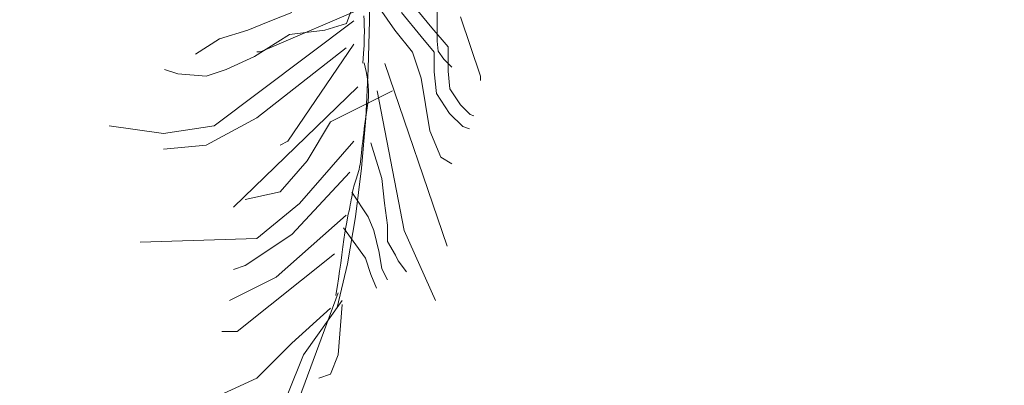
# Model space of a CAD drawing. Units: millimetres. Extents: x 595116 to 630915, y 909473 to 920225.
# Tile 57 of 134: x 629601.67 to 629608.928, y 919288.018 to 919290.711. Entities that reach past the tile are written whole.
import ezdxf

# ---------------------------------------------------------------- set-up
doc = ezdxf.new("R2010")
doc.units = ezdxf.units.MM
doc.layers.add('Dimension', color=3, linetype='Continuous', lineweight=18)
doc.layers.add('L-PLNT', color=85, linetype='Continuous', lineweight=13)
doc.styles.get("Standard").update_dxf_attribs({"font": 'arial.ttf'})
doc.dimstyles.new('ISO-25', dxfattribs={"dimtxt": 9, "dimasz": 6, "dimexe": 1.25, "dimexo": 0.625, "dimtad": 1, "dimlunit": 4, "dimtxsty": 'Standard', "dimcen": 2.5, "dimadec": 0, "dimazin": 0, "dimtfac": 1, "dimtmove": 0, "dimatfit": 3, "dimfxl": 1, "dimarcsym": 0})

# ---------------------------------------------------------------- blocks, each defined once
blk = doc.blocks.new('A$C4FB75ABC')
for p, q in [((3.3496, 1.0323), (3.3109, 0.9247)), ((3.3557, 1.0207), (3.3558, 0.9307)), ((3.3555, 0.9604), (3.142, 0.8689)), ((3.3755, 0.9548), (3.4056, 0.9118)), ((3.4413, 0.9609), (3.4779, 0.9162)), ((3.4889, 0.9539), (3.4889, 0.8899)), ((3.325, 0.9299), (3.0505, 0.7241)), ((3.1171, 0.9118), (3.1602, 0.929)), ((3.1602, 0.929), (3.2032, 0.9462)), ((3.3449, 0.9399), (3.3453, 0.931)), ((3.3453, 0.931), (3.3456, 0.921)), ((3.3558, 0.9307), (3.3535, 0.836)), ((3.4185, 0.9462), (3.4573, 0.8989)), ((3.5348, 0.9376), (3.5735, 0.8214)), ((3.0612, 0.8946), (3.1171, 0.9118)), ((3.2678, 0.9118), (3.1989, 0.9032)), ((3.3109, 0.9247), (3.2678, 0.9118)), ((3.3456, 0.921), (3.3457, 0.9097)), ((3.3457, 0.9097), (3.3456, 0.8969)), ((3.4056, 0.9118), (3.44, 0.8687)), ((3.4779, 0.9162), (3.5101, 0.8787)), ((3.0138, 0.8644), (3.0612, 0.8946)), ((3.1989, 0.9032), (3.1301, 0.8601)), ((3.3456, 0.8969), (3.3451, 0.8822)), ((3.4573, 0.8989), (3.4831, 0.8687)), ((3.4889, 0.8899), (3.4909, 0.8704)), ((3.3098, 0.8766), (3.1344, 0.7394)), ((3.325, 0.8842), (3.1954, 0.6936)), ((3.3451, 0.8822), (3.3441, 0.8655)), ((3.4909, 0.8704), (3.5015, 0.8546)), ((3.5101, 0.8787), (3.5101, 0.8314)), ((3.1301, 0.8601), (3.0741, 0.8343)), ((3.142, 0.8689), (3.1344, 0.8689)), ((3.3441, 0.8655), (3.3424, 0.8466)), ((3.44, 0.8687), (3.4573, 0.8171)), ((3.4831, 0.8687), (3.4831, 0.83)), ((3.5015, 0.8546), (3.5172, 0.8388)), ((2.9794, 0.8257), (2.9535, 0.8343)), ((3.0741, 0.8343), (3.0353, 0.8214)), ((3.3453, 0.8472), (3.3494, 0.8306)), ((3.3535, 0.836), (3.3484, 0.7387)), ((3.386, 0.8461), (3.508, 0.4878)), ((3.0353, 0.8214), (2.9794, 0.8257)), ((3.3494, 0.8306), (3.3521, 0.8161)), ((3.3521, 0.8161), (3.3535, 0.8034)), ((3.4573, 0.8171), (3.4659, 0.7655)), ((3.4831, 0.83), (3.4874, 0.787)), ((3.5101, 0.8314), (3.5136, 0.7963)), ((3.5735, 0.8214), (3.5735, 0.8128)), ((3.3326, 0.8003), (3.0886, 0.5641)), ((3.3535, 0.8034), (3.354, 0.7921)), ((3.5136, 0.7963), (3.5342, 0.7654)), ((3.4013, 0.7927), (3.2793, 0.7317)), ((3.3537, 0.7819), (3.3529, 0.7725)), ((3.354, 0.7921), (3.3537, 0.7819)), ((3.3708, 0.7927), (3.4242, 0.5183)), ((3.4874, 0.787), (3.5132, 0.7482)), ((3.3503, 0.7547), (3.349, 0.7457)), ((3.3517, 0.7635), (3.3503, 0.7547)), ((3.3529, 0.7725), (3.3517, 0.7635)), ((3.4659, 0.7655), (3.4745, 0.7138)), ((3.5342, 0.7654), (3.5536, 0.746)), ((3.1344, 0.7394), (3.0352, 0.686)), ((3.3484, 0.7387), (3.34, 0.641)), ((3.3478, 0.7367), (3.3466, 0.7276)), ((3.349, 0.7457), (3.3478, 0.7367)), ((3.5132, 0.7482), (3.5391, 0.7224)), ((3.5536, 0.746), (3.5605, 0.7437)), ((2.9513, 0.7089), (2.8446, 0.7241)), ((3.0505, 0.7241), (2.9513, 0.7089)), ((3.2793, 0.7317), (3.2335, 0.6555)), ((3.3455, 0.7186), (3.3445, 0.7097)), ((3.3466, 0.7276), (3.3455, 0.7186)), ((3.5391, 0.7224), (3.552, 0.7181)), ((3.3435, 0.7011), (3.3426, 0.6929)), ((3.3445, 0.7097), (3.3435, 0.7011)), ((3.4745, 0.7138), (3.496, 0.6622)), ((3.0352, 0.686), (2.9513, 0.6784)), ((3.1954, 0.6936), (3.1801, 0.686)), ((3.325, 0.6936), (3.2182, 0.5717)), ((3.341, 0.6779), (3.3402, 0.6711)), ((3.3417, 0.6851), (3.341, 0.6779)), ((3.3426, 0.6929), (3.3417, 0.6851)), ((3.3586, 0.6905), (3.3801, 0.6206)), ((3.3388, 0.6589), (3.338, 0.6533)), ((3.3395, 0.6648), (3.3388, 0.6589)), ((3.3402, 0.6711), (3.3395, 0.6648)), ((3.496, 0.6622), (3.5175, 0.6493)), ((3.2335, 0.6555), (3.1801, 0.5945)), ((3.34, 0.641), (3.3282, 0.5451)), ((3.3353, 0.6385), (3.3341, 0.634)), ((3.3363, 0.6432), (3.3353, 0.6385)), ((3.3372, 0.6481), (3.3363, 0.6432)), ((3.338, 0.6533), (3.3372, 0.6481)), ((3.3174, 0.6327), (3.203, 0.5107)), ((3.3303, 0.6215), (3.3289, 0.6175)), ((3.3316, 0.6256), (3.3303, 0.6215)), ((3.3329, 0.6297), (3.3316, 0.6256)), ((3.3341, 0.634), (3.3329, 0.6297)), ((3.3801, 0.6206), (3.3855, 0.5721)), ((3.3242, 0.6014), (3.3233, 0.5973)), ((3.3252, 0.6055), (3.3242, 0.6014)), ((3.3264, 0.6095), (3.3252, 0.6055)), ((3.3276, 0.6135), (3.3264, 0.6095)), ((3.3289, 0.6175), (3.3276, 0.6135)), ((3.1801, 0.5945), (3.1115, 0.5793)), ((3.3208, 0.584), (3.32, 0.5792)), ((3.3216, 0.5886), (3.3208, 0.584)), ((3.3209, 0.5936), (3.3532, 0.5452)), ((3.3225, 0.593), (3.3216, 0.5886)), ((3.3233, 0.5973), (3.3225, 0.593)), ((3.2182, 0.5717), (3.1344, 0.5031)), ((3.3169, 0.5634), (3.3156, 0.5574)), ((3.3181, 0.5689), (3.3169, 0.5634)), ((3.3191, 0.5742), (3.3181, 0.5689)), ((3.32, 0.5792), (3.3191, 0.5742)), ((3.3855, 0.5721), (3.3909, 0.5291)), ((3.3098, 0.5488), (3.1725, 0.4269)), ((3.3127, 0.5432), (3.3111, 0.5347)), ((3.3282, 0.5451), (3.3124, 0.4531)), ((3.3142, 0.5507), (3.3127, 0.5432)), ((3.3156, 0.5574), (3.3142, 0.5507)), ((3.3532, 0.5452), (3.364, 0.5183)), ((3.3047, 0.5237), (3.3478, 0.4645)), ((3.3093, 0.5249), (3.3075, 0.5137)), ((3.3111, 0.5347), (3.3093, 0.5249)), ((3.3909, 0.5291), (3.3909, 0.4968)), ((3.1344, 0.5031), (2.9056, 0.4955)), ((3.203, 0.5107), (3.1115, 0.4497)), ((3.3075, 0.5137), (3.3055, 0.5008)), ((3.364, 0.5183), (3.3747, 0.4753)), ((3.4242, 0.5183), (3.4852, 0.3811)), ((3.3034, 0.4863), (3.3013, 0.4707)), ((3.3055, 0.5008), (3.3034, 0.4863)), ((3.3909, 0.4968), (3.407, 0.4699)), ((3.2869, 0.4726), (3.0962, 0.3201)), ((3.3013, 0.4707), (3.2992, 0.4546)), ((3.3478, 0.4645), (3.3586, 0.4322)), ((3.3747, 0.4753), (3.3801, 0.443)), ((3.407, 0.4699), (3.4124, 0.4591)), ((3.1115, 0.4497), (3.0886, 0.4421)), ((3.3124, 0.4531), (3.2923, 0.3674)), ((3.2992, 0.4546), (3.297, 0.4387)), ((3.4124, 0.4591), (3.4286, 0.4376)), ((3.1725, 0.4269), (3.081, 0.3811)), ((3.297, 0.4387), (3.2949, 0.4237)), ((3.3586, 0.4322), (3.3693, 0.4053)), ((3.3801, 0.443), (3.3909, 0.4214)), ((3.2929, 0.4103), (3.2911, 0.3992)), ((3.2949, 0.4237), (3.2929, 0.4103)), ((3.2945, 0.3964), (3.2182, 0.1906)), ((3.2911, 0.3992), (3.2894, 0.3911)), ((3.3021, 0.3811), (3.2259, 0.2744)), ((3.3021, 0.3735), (3.2945, 0.2744)), ((3.2793, 0.3659), (3.203, 0.2973)), ((3.0962, 0.3201), (3.0657, 0.3201)), ((3.203, 0.2973), (3.1344, 0.2287)), ((3.2259, 0.2744), (3.1954, 0.1982)), ((3.2945, 0.2744), (3.2793, 0.2363)), ((3.2793, 0.2363), (3.2564, 0.2287)), ((3.1344, 0.2287), (3.0352, 0.1829))]:
    blk.add_line(p, q)
blk = doc.blocks.new('*D210')
at = {"layer": 'Defpoints', "color": 0, "transparency": 16777216}
for p in [(629586.2273, 919310.1229), (629593.9463, 919310.1229), (629586.2273, 919258.6624)]:
    blk.add_point(p, dxfattribs=at)
at = {"layer": 'Dimension', "color": 0, "lineweight": -2, "transparency": 16777216}
for p, q in [((629593.9463, 919310.1229), (629593.9463, 919449.6901)), ((629586.8523, 919310.1229), (629595.1963, 919310.1229)), ((629593.9463, 919264.6624), (629593.9463, 919304.1229)), ((629586.8523, 919258.6624), (629595.1963, 919258.6624))]:
    blk.add_line(p, q, dxfattribs=at)
at = {"layer": 'Dimension', "color": 0, "transparency": 16777216}
for points in [[(629592.9463, 919304.1229), (629594.9463, 919304.1229), (629593.9463, 919310.1229)], [(629592.9463, 919264.6624), (629594.9463, 919264.6624), (629593.9463, 919258.6624)]]:
    blk.add_solid(points, dxfattribs=at)
at = {"layer": 'Dimension', "color": 0, "transparency": 16777216, "insert": (629588.6617, 919382.9065), "char_height": 9, "attachment_point": 5, "rotation": 90}
blk.add_mtext('CANOPY 4\'-3 1/2" TYP.', dxfattribs=at)
blk = doc.blocks.new('*D216')
at = {"layer": 'Defpoints', "color": 0, "transparency": 16777216}
for p in [(629743.5408, 919411.9276), (629505.0408, 919411.8279), (629743.5408, 918832.3776)]:
    blk.add_point(p, dxfattribs=at)
at = {"layer": 'Dimension', "color": 0, "lineweight": -2, "transparency": 16777216}
for p, q in [((629743.5408, 919411.3026), (629743.5408, 918831.1276)), ((629505.0408, 919411.2029), (629505.0408, 918831.1276)), ((629511.0408, 918832.3776), (629737.5408, 918832.3776))]:
    blk.add_line(p, q, dxfattribs=at)
at = {"layer": 'Dimension', "color": 0, "transparency": 16777216}
for points in [[(629511.0408, 918833.3776), (629511.0408, 918831.3776), (629505.0408, 918832.3776)], [(629737.5408, 918833.3776), (629737.5408, 918831.3776), (629743.5408, 918832.3776)]]:
    blk.add_solid(points, dxfattribs=at)
at = {"layer": 'Dimension', "color": 0, "transparency": 16777216, "insert": (629624.2908, 918837.656), "char_height": 9, "attachment_point": 5}
blk.add_mtext('19\'-10 1/2"', dxfattribs=at)

msp = doc.modelspace()

# ---------------------------------------------------------------- block references
at = {"layer": 'L-PLNT', "xscale": 3.753413438031968, "yscale": 3.753413438031968, "zscale": 3.753413438031968}
msp.add_blockref('A$C4FB75ABC', (629591.6528, 919287.2124), dxfattribs=at)

# ---------------------------------------------------------------- dimensions: what is measured, and where the dimension line sits
at = {"layer": 'Dimension'}
dim = msp.add_linear_dim(base=(629593.9463, 919310.1229), p1=(629586.2273, 919258.6624), p2=(629586.2273, 919310.1229), angle=90, text='CANOPY <> TYP.', dimstyle='ISO-25', override={"dimdec": 1, "dimlfac": 1, "dimrnd": 0, "dimzin": 1, "dimdsep": 46, "dimlunit": 4, "dimfrac": 2}, dxfattribs=at)
dim.commit()
dim.dimension.update_dxf_attribs({"geometry": '*D210', "text_midpoint": (629588.6617, 919382.9065)})
dim = msp.add_linear_dim(base=(629743.5408, 918832.3776), p1=(629505.0408, 919411.8279), p2=(629743.5408, 919411.9276), dimstyle='ISO-25', override={"dimdec": 1, "dimlfac": 1, "dimrnd": 0, "dimzin": 1, "dimdsep": 46, "dimlunit": 4, "dimfrac": 2}, dxfattribs=at)
dim.commit()
dim.dimension.update_dxf_attribs({"geometry": '*D216', "text_midpoint": (629624.2908, 918837.656)})

doc.saveas('drawing.dxf')
